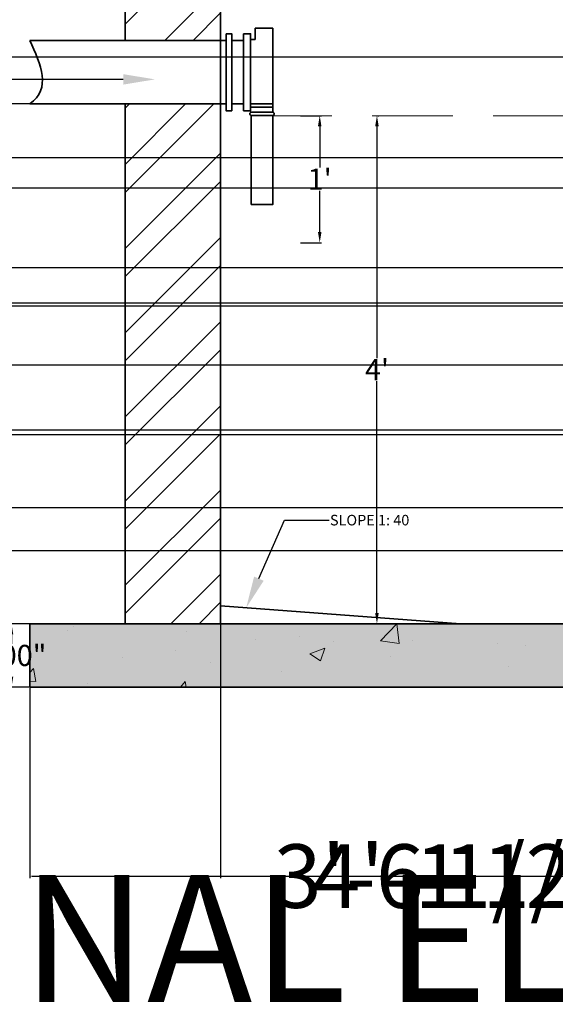
# Model space of a CAD drawing. Units: inches. Extents: x -34 to 285, y -151 to 155.
# Tile 2 of 10: x 22 to 72, y -151 to -58. Entities that reach past the tile are written whole.
import ezdxf
from ezdxf import colors
from ezdxf.entities.mleader import LeaderData, LeaderLine
from ezdxf.math import Vec2, Vec3

# ---------------------------------------------------------------- set-up
doc = ezdxf.new("R2010")
doc.units = ezdxf.units.IN
doc.header["$MEASUREMENT"] = 0
doc.linetypes.add('DASHED', pattern=[19.05, 12.7, -6.35])
for name, color, linetype, lineweight in [('A-ANNO-DIMS', 2, 'Continuous', 18), ('A-ANNO-TEXT', 7, 'Continuous', 25), ('A-DETL', 7, 'Continuous', 35), ('A-DETL-HIDN', 8, 'DASHED', 18), ('A-DETL-PATT', 8, 'Continuous', 18), ('P-SANR-PATT', 8, 'Continuous', 13), ('P-SANR-PIPE', 4, 'Continuous', 35)]:
    doc.layers.add(name, color=color, linetype=linetype, lineweight=lineweight)
doc.styles.get("Standard").update_dxf_attribs({"font": 'arial.ttf'})
doc.dimstyles.get("Standard").update_dxf_attribs({"dimtxt": 6, "dimasz": 0.18, "dimexe": 0.18, "dimexo": 0.0625, "dimgap": 0.09, "dimtad": 0, "dimtih": 1, "dimtoh": 1, "dimzin": 0, "dimdsep": 46, "dimlunit": 3, "dimtxsty": 'Standard', "dimcen": 0.09, "dimadec": 0, "dimazin": 0, "dimtfac": 1, "dimtofl": 0, "dimtmove": 0, "dimatfit": 3, "dimfxl": 1, "dimtolj": 1, "dimtzin": 0, "dimarcsym": 0})
pattern_1 = [(50, (9.538, 3.616), (14.3452, -1.255), [1.5, -16.5]), (355, (9.538, 3.616), (-2.775, 15.0438), [1.2, -13.2]), (100.451, (10.733, 3.511), (11.5702, 13.7888), [1.2748, -14.0228]), (46.184, (9.538, 7.616), (21.345, -3.3104), [2.25, -24.75]), (96.636, (11.317, 7.34), (18.693, 19.4824), [1.912, -21.0343]), (351.184, (9.538, 7.616), (18.693, 19.4824), [1.8, -19.8]), (21, (11.538, 6.616), (11.9381, -8.0524), [1.5, -16.5]), (326, (11.538, 6.616), (4.8663, 14.503), [1.2, -13.2]), (71.451, (12.533, 5.945), (16.8044, 6.4506), [1.2748, -14.0228]), (37.5, (9.538, 3.616), (0.2432, 6.65788), [0, -13.04, 0, -13.4, 0, -13.25]), (7.5, (9.538, 3.616), (5.2614, 7.88823), [0, -7.64, 0, -12.74, 0, -5.05]), (327.5, (5.078, 3.616), (10.67645, -0.4511), [0, -5, 0, -15.6, 0, -20.7]), (317.5, (3.078, 3.616), (11.6637, 2.0021), [0, -6.5, 0, -10.36, 0, -14.7])]

# ---------------------------------------------------------------- blocks, each defined once
blk = doc.blocks.new('*D26')
at = {"layer": 'A-ANNO-DIMS', "color": 0, "lineweight": -2, "transparency": 16777216}
for p, q in [((48.419, -66.969), (50.405, -66.969)), ((50.225, -67.969), (50.225, -71.875)), ((50.225, -77.969), (50.225, -74.063)), ((48.419, -78.969), (50.405, -78.969))]:
    blk.add_line(p, q, dxfattribs=at)
at = {"layer": 'A-ANNO-DIMS', "color": 0, "transparency": 16777216}
for points in [[(50.058, -67.969), (50.391, -67.969), (50.225, -66.969)], [(50.058, -77.969), (50.391, -77.969), (50.225, -78.969)]]:
    blk.add_solid(points, dxfattribs=at)
at = {"layer": 'Defpoints', "color": 0, "transparency": 16777216}
for p in [(48.356, -66.969), (48.356, -78.969), (50.225, -78.969)]:
    blk.add_point(p, dxfattribs=at)
at = {"layer": 'A-ANNO-DIMS', "color": 0, "transparency": 16777216, "insert": (50.225, -72.969), "char_height": 2, "attachment_point": 5}
blk.add_mtext("\\A1;1'", dxfattribs=at)
blk = doc.blocks.new('*D27')
at = {"layer": 'A-ANNO-DIMS', "color": 0, "lineweight": -2, "transparency": 16777216}
for p, q in [((55.697, -66.969), (55.814, -66.969)), ((55.634, -67.969), (55.634, -89.879)), ((55.634, -113.969), (55.634, -92.059)), ((55.697, -114.969), (55.814, -114.969))]:
    blk.add_line(p, q, dxfattribs=at)
at = {"layer": 'A-ANNO-DIMS', "color": 0, "transparency": 16777216}
for points in [[(55.468, -67.969), (55.801, -67.969), (55.634, -66.969)], [(55.468, -113.969), (55.801, -113.969), (55.634, -114.969)]]:
    blk.add_solid(points, dxfattribs=at)
at = {"layer": 'Defpoints', "color": 0, "transparency": 16777216}
for p in [(55.634, -66.969), (55.634, -114.969), (55.634, -114.969)]:
    blk.add_point(p, dxfattribs=at)
at = {"layer": 'A-ANNO-DIMS', "color": 0, "transparency": 16777216, "insert": (55.634, -90.969), "char_height": 2, "attachment_point": 5}
blk.add_mtext("\\A1;4'", dxfattribs=at)
blk = doc.blocks.new('*D35')
at = {"layer": 'A-ANNO-DIMS', "color": 0, "lineweight": -2, "transparency": 16777216}
for p, q in [((21.5, -42.969), (13.144, -42.969)), ((13.324, -43.969), (13.324, -80.858)), ((13.324, -119.969), (13.324, -83.08)), ((22.783, -120.969), (13.144, -120.969))]:
    blk.add_line(p, q, dxfattribs=at)
at = {"layer": 'A-ANNO-DIMS', "color": 0, "transparency": 16777216}
for points in [[(13.157, -43.969), (13.491, -43.969), (13.324, -42.969)], [(13.157, -119.969), (13.491, -119.969), (13.324, -120.969)]]:
    blk.add_solid(points, dxfattribs=at)
at = {"layer": 'Defpoints', "color": 0, "transparency": 16777216}
for p in [(13.324, -42.969), (21.563, -42.969), (22.846, -120.969)]:
    blk.add_point(p, dxfattribs=at)
at = {"layer": 'A-ANNO-DIMS', "color": 0, "transparency": 16777216, "insert": (13.324, -81.969), "char_height": 2, "attachment_point": 5}
blk.add_mtext('\\A1;6\'-6.00"', dxfattribs=at)
blk = doc.blocks.new('*D37')
at = {"layer": 'A-ANNO-DIMS', "color": 0, "lineweight": -2, "transparency": 16777216}
for p, q in [((22.783, -114.969), (20.931, -114.969)), ((21.111, -115.969), (21.111, -116.858)), ((21.111, -119.969), (21.111, -119.08)), ((22.783, -120.969), (20.931, -120.969))]:
    blk.add_line(p, q, dxfattribs=at)
at = {"layer": 'A-ANNO-DIMS', "color": 0, "transparency": 16777216}
for points in [[(20.944, -115.969), (21.278, -115.969), (21.111, -114.969)], [(20.944, -119.969), (21.278, -119.969), (21.111, -120.969)]]:
    blk.add_solid(points, dxfattribs=at)
at = {"layer": 'Defpoints', "color": 0, "transparency": 16777216}
for p in [(22.846, -114.969), (21.111, -120.969), (22.846, -120.969)]:
    blk.add_point(p, dxfattribs=at)
at = {"layer": 'A-ANNO-DIMS', "color": 0, "transparency": 16777216, "insert": (21.111, -117.969), "char_height": 2, "attachment_point": 5}
blk.add_mtext('\\A1;6.00"', dxfattribs=at)
blk = doc.blocks.new('PIPE-SOCKET')
for p, q in [((1.802, 8.25), (0.129, 8.25)), ((1.802, 7.168), (1.802, 8.25)), ((2.233, 7.168), (1.802, 7.168)), ((2.233, 7.168), (2.233, 7.168))]:
    blk.add_line(p, q)
for points in [[(0.129, 0.312), (0.129, 8.25), (1.802, 8.25)], [(0.129, 0.312), (2.172, 0.312)]]:
    blk.add_lwpolyline(points)
for centre, start, end in [((0.157, 0.157), 100.54101, 280.54101), ((2.144, 0.157), 259.45899, 79.45899)]:
    blk.add_arc(centre, 0.157, start, end)
blk = doc.blocks.new('*D48')
at = {"layer": 'A-ANNO-DIMS', "color": 0, "lineweight": -2, "transparency": 16777216}
for p, q in [((22.846, -121.031), (22.846, -138.999)), ((214.846, -121.031), (214.846, -138.999)), ((23.026, -138.819), (108.733, -138.819)), ((214.666, -138.819), (128.959, -138.819))]:
    blk.add_line(p, q, dxfattribs=at)
at = {"layer": 'A-ANNO-DIMS', "color": 0, "transparency": 16777216}
for points in [[(23.026, -138.789), (23.026, -138.849), (22.846, -138.819)], [(214.666, -138.789), (214.666, -138.849), (214.846, -138.819)]]:
    blk.add_solid(points, dxfattribs=at)
at = {"layer": 'Defpoints', "color": 0, "transparency": 16777216}
for p in [(22.846, -120.969), (214.846, -120.969), (214.846, -138.819)]:
    blk.add_point(p, dxfattribs=at)
at = {"layer": 'A-ANNO-DIMS', "color": 0, "transparency": 16777216, "insert": (118.846, -138.819), "char_height": 6, "attachment_point": 5}
blk.add_mtext('\\A1;16\'-0"', dxfattribs=at)
blk = doc.blocks.new('*D57')
at = {"layer": 'A-ANNO-DIMS', "color": 0, "lineweight": -2, "transparency": 16777216}
for p, q in [((41.321, -65.853), (0.722, -65.853)), ((0.902, -66.033), (0.902, -87.309)), ((0.902, -114.789), (0.902, -93.513)), ((40.783, -114.969), (0.722, -114.969))]:
    blk.add_line(p, q, dxfattribs=at)
at = {"layer": 'A-ANNO-DIMS', "color": 0, "transparency": 16777216}
for points in [[(0.872, -66.033), (0.932, -66.033), (0.902, -65.853)], [(0.872, -114.789), (0.932, -114.789), (0.902, -114.969)]]:
    blk.add_solid(points, dxfattribs=at)
at = {"layer": 'Defpoints', "color": 0, "transparency": 16777216}
for p in [(41.384, -65.853), (0.902, -114.969), (40.846, -114.969)]:
    blk.add_point(p, dxfattribs=at)
at = {"layer": 'A-ANNO-DIMS', "color": 0, "transparency": 16777216, "insert": (0.902, -90.411), "char_height": 6, "attachment_point": 5}
blk.add_mtext('\\A1;4\'-1"', dxfattribs=at)
blk = doc.blocks.new('*D58')
at = {"layer": 'A-ANNO-DIMS', "color": 0, "lineweight": -2, "transparency": 16777216}
for p, q in [((83.099, -61.477), (83.099, -138.999)), ((40.846, -115.031), (40.846, -138.999)), ((41.026, -138.819), (46.919, -138.819)), ((82.919, -138.819), (77.026, -138.819))]:
    blk.add_line(p, q, dxfattribs=at)
at = {"layer": 'A-ANNO-DIMS', "color": 0, "transparency": 16777216}
for points in [[(41.026, -138.789), (41.026, -138.849), (40.846, -138.819)], [(82.919, -138.789), (82.919, -138.849), (83.099, -138.819)]]:
    blk.add_solid(points, dxfattribs=at)
at = {"layer": 'Defpoints', "color": 0, "transparency": 16777216}
for p in [(83.099, -61.415), (40.846, -114.969), (83.099, -138.819)]:
    blk.add_point(p, dxfattribs=at)
at = {"layer": 'A-ANNO-DIMS', "color": 0, "transparency": 16777216, "insert": (61.973, -138.819), "char_height": 6, "attachment_point": 5}
blk.add_mtext('\\A1;3\'-6 1/2"', dxfattribs=at)
blk = doc.blocks.new('*D60')
at = {"layer": 'A-ANNO-DIMS', "color": 0, "lineweight": -2, "transparency": 16777216}
for p, q in [((90.383, -71.009), (90.383, -138.999)), ((40.846, -115.031), (40.846, -138.999)), ((41.026, -138.819), (50.439, -138.819)), ((90.203, -138.819), (80.791, -138.819))]:
    blk.add_line(p, q, dxfattribs=at)
at = {"layer": 'A-ANNO-DIMS', "color": 0, "transparency": 16777216}
for points in [[(41.026, -138.789), (41.026, -138.849), (40.846, -138.819)], [(90.203, -138.789), (90.203, -138.849), (90.383, -138.819)]]:
    blk.add_solid(points, dxfattribs=at)
at = {"layer": 'Defpoints', "color": 0, "transparency": 16777216}
for p in [(90.383, -70.947), (40.846, -114.969), (90.383, -138.819)]:
    blk.add_point(p, dxfattribs=at)
at = {"layer": 'A-ANNO-DIMS', "color": 0, "transparency": 16777216, "insert": (65.615, -138.819), "char_height": 6, "attachment_point": 5}
blk.add_mtext('\\A1;4\'-1 1/2"', dxfattribs=at)
blk = doc.blocks.new('*D64')
at = {"layer": 'A-ANNO-DIMS', "color": 0, "lineweight": -2, "transparency": 16777216}
for p, q in [((157.783, -84.969), (0.722, -84.969)), ((0.902, -85.149), (0.902, -96.816)), ((0.902, -114.789), (0.902, -103.122)), ((148.783, -114.969), (0.722, -114.969))]:
    blk.add_line(p, q, dxfattribs=at)
at = {"layer": 'A-ANNO-DIMS', "color": 0, "transparency": 16777216}
for points in [[(0.872, -85.149), (0.932, -85.149), (0.902, -84.969)], [(0.872, -114.789), (0.932, -114.789), (0.902, -114.969)]]:
    blk.add_solid(points, dxfattribs=at)
at = {"layer": 'Defpoints', "color": 0, "transparency": 16777216}
for p in [(157.846, -84.969), (0.902, -114.969), (148.846, -114.969)]:
    blk.add_point(p, dxfattribs=at)
at = {"layer": 'A-ANNO-DIMS', "color": 0, "transparency": 16777216, "insert": (0.902, -99.969), "char_height": 6, "attachment_point": 5}
blk.add_mtext('\\A1;2\'-6"', dxfattribs=at)
blk = doc.blocks.new('*D67')
at = {"layer": 'A-ANNO-DIMS', "color": 0, "lineweight": -2, "transparency": 16777216}
for p, q in [((90.321, -70.947), (0.722, -70.947)), ((0.902, -71.127), (0.902, -89.802)), ((0.902, -114.789), (0.902, -96.113)), ((118.783, -114.969), (0.722, -114.969))]:
    blk.add_line(p, q, dxfattribs=at)
at = {"layer": 'A-ANNO-DIMS', "color": 0, "transparency": 16777216}
for points in [[(0.872, -71.127), (0.932, -71.127), (0.902, -70.947)], [(0.872, -114.789), (0.932, -114.789), (0.902, -114.969)]]:
    blk.add_solid(points, dxfattribs=at)
at = {"layer": 'Defpoints', "color": 0, "transparency": 16777216}
for p in [(90.383, -70.947), (0.902, -114.969), (118.846, -114.969)]:
    blk.add_point(p, dxfattribs=at)
at = {"layer": 'A-ANNO-DIMS', "color": 0, "transparency": 16777216, "insert": (0.902, -92.958), "char_height": 6, "attachment_point": 5}
blk.add_mtext('\\A1;3\'-8"', dxfattribs=at)
blk = doc.blocks.new('*D72')
at = {"layer": 'A-ANNO-DIMS', "color": 0, "lineweight": -2, "transparency": 16777216}
for p, q in [((90.321, -70.947), (0.722, -70.947)), ((0.902, -71.127), (0.902, -72.953)), ((0.902, -81.165), (0.902, -79.338)), ((97.605, -81.345), (0.722, -81.345))]:
    blk.add_line(p, q, dxfattribs=at)
at = {"layer": 'A-ANNO-DIMS', "color": 0, "transparency": 16777216}
for points in [[(0.872, -71.127), (0.932, -71.127), (0.902, -70.947)], [(0.872, -81.165), (0.932, -81.165), (0.902, -81.345)]]:
    blk.add_solid(points, dxfattribs=at)
at = {"layer": 'Defpoints', "color": 0, "transparency": 16777216}
for p in [(90.383, -70.947), (0.902, -81.345), (97.668, -81.345)]:
    blk.add_point(p, dxfattribs=at)
at = {"layer": 'A-ANNO-DIMS', "color": 0, "transparency": 16777216, "insert": (0.902, -76.146), "char_height": 6, "attachment_point": 5}
blk.add_mtext('\\A1;0\'-10 1/2"', dxfattribs=at)
blk = doc.blocks.new('*D73')
at = {"layer": 'A-ANNO-DIMS', "color": 0, "lineweight": -2, "transparency": 16777216}
for p, q in [((97.605, -81.345), (0.722, -81.345)), ((0.902, -81.525), (0.902, -82.784)), ((0.902, -90.35), (0.902, -89.091)), ((105.236, -90.53), (0.722, -90.53))]:
    blk.add_line(p, q, dxfattribs=at)
at = {"layer": 'A-ANNO-DIMS', "color": 0, "transparency": 16777216}
for points in [[(0.872, -81.525), (0.932, -81.525), (0.902, -81.345)], [(0.872, -90.35), (0.932, -90.35), (0.902, -90.53)]]:
    blk.add_solid(points, dxfattribs=at)
at = {"layer": 'Defpoints', "color": 0, "transparency": 16777216}
for p in [(97.668, -81.345), (0.902, -90.53), (105.299, -90.53)]:
    blk.add_point(p, dxfattribs=at)
at = {"layer": 'A-ANNO-DIMS', "color": 0, "transparency": 16777216, "insert": (0.902, -85.937), "char_height": 6, "attachment_point": 5}
blk.add_mtext('\\A1;0\'-9"', dxfattribs=at)
blk = doc.blocks.new('*D74')
at = {"layer": 'A-ANNO-DIMS', "color": 0, "lineweight": -2, "transparency": 16777216}
for p, q in [((0.902, -90.35), (0.902, -90.17)), ((105.236, -90.53), (0.722, -90.53)), ((115.989, -97.116), (0.722, -97.116)), ((0.902, -97.296), (0.902, -97.476))]:
    blk.add_line(p, q, dxfattribs=at)
at = {"layer": 'A-ANNO-DIMS', "color": 0, "transparency": 16777216}
for points in [[(0.872, -90.35), (0.932, -90.35), (0.902, -90.53)], [(0.872, -97.296), (0.932, -97.296), (0.902, -97.116)]]:
    blk.add_solid(points, dxfattribs=at)
at = {"layer": 'Defpoints', "color": 0, "transparency": 16777216}
for p in [(105.299, -90.53), (0.902, -97.116), (116.051, -97.116)]:
    blk.add_point(p, dxfattribs=at)
at = {"layer": 'A-ANNO-DIMS', "color": 0, "transparency": 16777216, "insert": (0.902, -93.823), "char_height": 6, "attachment_point": 5}
blk.add_mtext('\\A1;0\'-6 1/2"', dxfattribs=at)
blk = doc.blocks.new('*D75')
at = {"layer": 'A-ANNO-DIMS', "color": 0, "lineweight": -2, "transparency": 16777216}
for p, q in [((115.989, -97.116), (0.722, -97.116)), ((0.902, -97.296), (0.902, -97.419)), ((121.836, -104.028), (0.722, -104.028)), ((0.902, -103.848), (0.902, -103.725))]:
    blk.add_line(p, q, dxfattribs=at)
at = {"layer": 'A-ANNO-DIMS', "color": 0, "transparency": 16777216}
for points in [[(0.872, -97.296), (0.932, -97.296), (0.902, -97.116)], [(0.872, -103.848), (0.932, -103.848), (0.902, -104.028)]]:
    blk.add_solid(points, dxfattribs=at)
at = {"layer": 'Defpoints', "color": 0, "transparency": 16777216}
for p in [(116.051, -97.116), (0.902, -104.028), (121.899, -104.028)]:
    blk.add_point(p, dxfattribs=at)
at = {"layer": 'A-ANNO-DIMS', "color": 0, "transparency": 16777216, "insert": (0.902, -100.572), "char_height": 6, "attachment_point": 5}
blk.add_mtext('\\A1;0\'-7"', dxfattribs=at)
blk = doc.blocks.new('*D76')
at = {"layer": 'A-ANNO-DIMS', "color": 0, "lineweight": -2, "transparency": 16777216}
for p, q in [((121.836, -104.028), (0.722, -104.028)), ((0.902, -104.208), (0.902, -106.345)), ((0.902, -114.789), (0.902, -112.652)), ((118.783, -114.969), (0.722, -114.969))]:
    blk.add_line(p, q, dxfattribs=at)
at = {"layer": 'A-ANNO-DIMS', "color": 0, "transparency": 16777216}
for points in [[(0.872, -104.208), (0.932, -104.208), (0.902, -104.028)], [(0.872, -114.789), (0.932, -114.789), (0.902, -114.969)]]:
    blk.add_solid(points, dxfattribs=at)
at = {"layer": 'Defpoints', "color": 0, "transparency": 16777216}
for p in [(121.899, -104.028), (0.902, -114.969), (118.846, -114.969)]:
    blk.add_point(p, dxfattribs=at)
at = {"layer": 'A-ANNO-DIMS', "color": 0, "transparency": 16777216, "insert": (0.902, -109.499), "char_height": 6, "attachment_point": 5}
blk.add_mtext('\\A1;0\'-11"', dxfattribs=at)
blk = doc.blocks.new('*D83')
at = {"layer": 'A-ANNO-DIMS', "color": 0, "lineweight": -2, "transparency": 16777216}
for p, q in [((153.652, -61.451), (0.722, -61.451)), ((0.902, -61.631), (0.902, -64.435)), ((0.902, -73.623), (0.902, -70.819)), ((162.652, -73.803), (0.722, -73.803))]:
    blk.add_line(p, q, dxfattribs=at)
at = {"layer": 'A-ANNO-DIMS', "color": 0, "transparency": 16777216}
for points in [[(0.872, -61.631), (0.932, -61.631), (0.902, -61.451)], [(0.872, -73.623), (0.932, -73.623), (0.902, -73.803)]]:
    blk.add_solid(points, dxfattribs=at)
at = {"layer": 'Defpoints', "color": 0, "transparency": 16777216}
for p in [(153.715, -61.451), (0.902, -73.803), (162.715, -73.803)]:
    blk.add_point(p, dxfattribs=at)
at = {"layer": 'A-ANNO-DIMS', "color": 0, "transparency": 16777216, "insert": (0.902, -67.627), "char_height": 6, "attachment_point": 5}
blk.add_mtext('\\A1;1\'-0 1/2"', dxfattribs=at)
blk = doc.blocks.new('*D84')
at = {"layer": 'A-ANNO-DIMS', "color": 0, "lineweight": -2, "transparency": 16777216}
for p, q in [((162.652, -73.803), (0.722, -73.803)), ((0.902, -73.983), (0.902, -76.094)), ((0.902, -84.513), (0.902, -82.401)), ((169.24, -84.693), (0.722, -84.693))]:
    blk.add_line(p, q, dxfattribs=at)
at = {"layer": 'A-ANNO-DIMS', "color": 0, "transparency": 16777216}
for points in [[(0.872, -73.983), (0.932, -73.983), (0.902, -73.803)], [(0.872, -84.513), (0.932, -84.513), (0.902, -84.693)]]:
    blk.add_solid(points, dxfattribs=at)
at = {"layer": 'Defpoints', "color": 0, "transparency": 16777216}
for p in [(162.715, -73.803), (0.902, -84.693), (169.303, -84.693)]:
    blk.add_point(p, dxfattribs=at)
at = {"layer": 'A-ANNO-DIMS', "color": 0, "transparency": 16777216, "insert": (0.902, -79.248), "char_height": 6, "attachment_point": 5}
blk.add_mtext('\\A1;0\'-11"', dxfattribs=at)
blk = doc.blocks.new('*D85')
at = {"layer": 'A-ANNO-DIMS', "color": 0, "lineweight": -2, "transparency": 16777216}
for p, q in [((169.24, -84.693), (0.722, -84.693)), ((0.902, -84.873), (0.902, -87.539)), ((0.902, -96.513), (0.902, -93.846)), ((179.419, -96.693), (0.722, -96.693))]:
    blk.add_line(p, q, dxfattribs=at)
at = {"layer": 'A-ANNO-DIMS', "color": 0, "transparency": 16777216}
for points in [[(0.872, -84.873), (0.932, -84.873), (0.902, -84.693)], [(0.872, -96.513), (0.932, -96.513), (0.902, -96.693)]]:
    blk.add_solid(points, dxfattribs=at)
at = {"layer": 'Defpoints', "color": 0, "transparency": 16777216}
for p in [(169.303, -84.693), (0.902, -96.693), (179.482, -96.693)]:
    blk.add_point(p, dxfattribs=at)
at = {"layer": 'A-ANNO-DIMS', "color": 0, "transparency": 16777216, "insert": (0.902, -90.693), "char_height": 6, "attachment_point": 5}
blk.add_mtext('\\A1;1\'-0"', dxfattribs=at)
blk = doc.blocks.new('*D86')
at = {"layer": 'A-ANNO-DIMS', "color": 0, "lineweight": -2, "transparency": 16777216}
for p, q in [((179.419, -96.693), (0.722, -96.693)), ((0.902, -96.873), (0.902, -99.189)), ((0.902, -107.89), (0.902, -105.574)), ((187.783, -108.07), (0.722, -108.07))]:
    blk.add_line(p, q, dxfattribs=at)
at = {"layer": 'A-ANNO-DIMS', "color": 0, "transparency": 16777216}
for points in [[(0.872, -96.873), (0.932, -96.873), (0.902, -96.693)], [(0.872, -107.89), (0.932, -107.89), (0.902, -108.07)]]:
    blk.add_solid(points, dxfattribs=at)
at = {"layer": 'Defpoints', "color": 0, "transparency": 16777216}
for p in [(179.482, -96.693), (0.902, -108.07), (187.846, -108.07)]:
    blk.add_point(p, dxfattribs=at)
at = {"layer": 'A-ANNO-DIMS', "color": 0, "transparency": 16777216, "insert": (0.902, -102.381), "char_height": 6, "attachment_point": 5}
blk.add_mtext('\\A1;0\'-11 1/2"', dxfattribs=at)
blk = doc.blocks.new('*D87')
at = {"layer": 'A-ANNO-DIMS', "color": 0, "lineweight": -2, "transparency": 16777216}
for p, q in [((187.783, -108.07), (0.722, -108.07)), ((0.902, -108.25), (0.902, -108.366)), ((196.783, -114.969), (0.722, -114.969)), ((0.902, -114.789), (0.902, -114.673))]:
    blk.add_line(p, q, dxfattribs=at)
at = {"layer": 'A-ANNO-DIMS', "color": 0, "transparency": 16777216}
for points in [[(0.872, -108.25), (0.932, -108.25), (0.902, -108.07)], [(0.872, -114.789), (0.932, -114.789), (0.902, -114.969)]]:
    blk.add_solid(points, dxfattribs=at)
at = {"layer": 'Defpoints', "color": 0, "transparency": 16777216}
for p in [(187.846, -108.07), (0.902, -114.969), (196.846, -114.969)]:
    blk.add_point(p, dxfattribs=at)
at = {"layer": 'A-ANNO-DIMS', "color": 0, "transparency": 16777216, "insert": (0.902, -111.519), "char_height": 6, "attachment_point": 5}
blk.add_mtext('\\A1;0\'-7"', dxfattribs=at)

msp = doc.modelspace()

# ---------------------------------------------------------------- hatches: boundary and pattern name
at = {"layer": 'A-DETL-PATT'}
h = msp.add_hatch(dxfattribs=at)
h.set_pattern_fill('AR-CONC', color=256, scale=0.4)
h.set_pattern_definition([(50, (0, 0), (2.86904, -0.251009), [0.3, -3.3]), (355, (0, 0), (-0.555005, 3.00877), [0.24, -2.64]), (100.4514, (0.239, -0.021), (2.314035, 2.75776), [0.25496, -2.80457]), (46.1842, (0, 0.8), (4.268965, -0.662077), [0.45, -4.95]), (96.6356, (0.3557, 0.745), (3.73865, 3.896474), [0.38244, -4.206855]), (351.1842, (0, 0.8), (3.73865, 3.896474), [0.36, -3.96]), (21, (0.4, 0.6), (2.387628, -1.610476), [0.3, -3.3]), (326, (0.4, 0.6), (0.97326, 2.9006), [0.24, -2.64]), (71.4514, (0.599, 0.4658), (3.36089, 1.290125), [0.25496, -2.80457]), (37.5, (0, 0), (0.0486394, 1.3315754), [0, -2.608, 0, -2.68, 0, -2.65]), (7.5, (0, 0), (1.052278, 1.577647), [0, -1.528, 0, -2.548, 0, -1.01]), (327.5, (-0.892, 0), (2.1352897, -0.0902195), [0, -1, 0, -3.12, 0, -4.14]), (317.5, (-1.292, 0), (2.332745, 0.40042), [0, -1.3, 0, -2.072, 0, -2.94])])
h.paths.add_polyline_path([(214.846, -48.969), (214.846, -42.969), (184.518, -42.969), (184.518, -48.969)])
h.paths.add_polyline_path([(122.241, -42.969), (122.241, -48.969), (155.156, -48.969), (155.156, -42.969)])
h.paths.add_polyline_path([(214.846, -114.969), (22.846, -114.969), (22.846, -120.969), (214.846, -120.969)])
h = msp.add_hatch(dxfattribs=at)
h.set_pattern_fill('ANSI32', color=256, scale=15)
h.paths.add_polyline_path([(148.846, -59.969), (139.846, -59.969), (139.846, -66.969), (148.846, -66.969)])
h.paths.add_polyline_path([(148.846, -66.969), (139.846, -66.969), (139.846, -78.969), (148.846, -78.969)])
h.paths.add_polyline_path([(148.846, -84.969), (139.846, -84.969), (139.846, -85.88), (139.846, -114.969), (148.846, -114.969)])
h.paths.add_polyline_path([(40.846, -65.853), (32.384, -65.853), (31.846, -65.853), (31.846, -114.969), (40.846, -114.969)])
h.paths.add_polyline_path([(40.846, -48.969), (31.846, -48.969), (31.846, -59.853), (40.846, -59.853)])
h = msp.add_hatch(dxfattribs=at)
h.set_pattern_fill('AR-CONC', color=256, scale=2)
h.paths.add_polyline_path([(22.846, -114.969), (22.846, -120.969), (214.846, -120.969), (214.846, -114.969)])
at = {"layer": 'P-SANR-PATT'}
h = msp.add_hatch(dxfattribs=at)
h.set_pattern_fill('AR-CONC', color=256, scale=2)
h.set_pattern_definition(pattern_1)
h.paths.add_polyline_path([(41.921, -59.235), (41.384, -59.235), (41.384, -66.504), (41.921, -66.504)])
h.paths.add_polyline_path([(43.693, -59.235), (43.04, -59.235), (43.04, -66.504), (43.693, -66.504)])
h = msp.add_hatch(dxfattribs=at)
h.set_pattern_fill('AR-CONC', color=256, scale=2)
h.set_pattern_definition(pattern_1)
h.paths.add_polyline_path([(45.798, -66.948, 0.831086), (45.798, -66.639), (43.754, -66.639, 0.831086), (43.754, -66.948)])
h = msp.add_hatch(dxfattribs=at)
h.set_pattern_fill('AR-CONC', color=256, scale=2)
h.paths.add_polyline_path([(34.155, -69.469), (36.26, -69.469), (36.26, -69.778), (34.155, -69.778)])

# ---------------------------------------------------------------- linework, layer by layer
at = {"layer": 'A-DETL'}
for p, q in [((31.846, -48.969), (31.846, -59.853)), ((40.846, -48.969), (40.846, -114.969)), ((31.846, -65.853), (31.846, -114.969)), ((40.846, -113.284), (63.519, -114.969)), ((22.846, -114.969), (22.846, -120.969)), ((22.846, -114.969), (214.846, -114.969)), ((22.846, -120.969), (214.846, -120.969))]:
    msp.add_line(p, q, dxfattribs=at)
at = {"layer": 'A-DETL-HIDN', "ltscale": 0.6}
msp.add_line((43.754, -66.969), (73.547, -66.969), dxfattribs=at)
at = {"layer": 'P-SANR-PIPE'}
for p, q in [((41.384, -59.853), (22.832, -59.853)), ((41.384, -59.853), (32.384, -59.853)), ((41.384, -65.853), (22.832, -65.853)), ((41.384, -65.853), (23.384, -65.853)), ((41.384, -65.853), (32.384, -65.853)), ((43.04, -65.853), (41.921, -65.853)), ((45.798, -75.353), (43.754, -75.353))]:
    msp.add_line(p, q, dxfattribs=at)
for points in [[(41.384, -59.235), (41.921, -59.235), (41.921, -66.504), (41.384, -66.504)], [(43.04, -59.235), (43.693, -59.235), (43.693, -66.504), (43.04, -66.504)], [(41.921, -59.853), (43.04, -59.853), (43.04, -65.853), (41.921, -65.853)]]:
    msp.add_lwpolyline(points, close=True, dxfattribs=at)
for points in [[(32.384, -59.853), (22.832, -59.853)], [(22.832, -65.853), (32.384, -65.853)], [(43.693, -66.162), (45.798, -66.162), (45.798, -65.853), (43.754, -65.853)], [(43.754, -66.948), (43.754, -75.353), (45.798, -75.353), (45.798, -66.948)], [(43.754, -66.948), (45.798, -66.948)]]:
    msp.add_lwpolyline(points, dxfattribs=at)
msp.add_open_spline([(22.832, -59.853), (23.874, -62.138), (24.916, -64.424), (22.832, -65.853)], degree=3, dxfattribs=at)

# ---------------------------------------------------------------- block references
at = {"layer": 'P-SANR-PIPE', "extrusion": (0, 0, -1), "zscale": -1}
msp.add_blockref('PIPE-SOCKET', (-45.926, -66.951), dxfattribs=at)

# ---------------------------------------------------------------- texts
at = {"layer": 'A-ANNO-TEXT', "insert": (-34.52, -138.72), "char_height": 12, "attachment_point": 1}
msp.add_mtext_dynamic_manual_height_columns('SECTIONAL ELEVATION OF A SEPTIC TANK ', width=509.35271, gutter_width=1, heights=[0], dxfattribs=at)

# ---------------------------------------------------------------- dimensions: what is measured, and where the dimension line sits
at = {"layer": 'A-ANNO-DIMS'}
for base, p1, p2, override, picture, middle in [((13.324, -42.969), (22.846, -120.969), (21.563, -42.969), {"dimtxt": 2, "dimasz": 1, "dimclrd": 0, "dimclre": 0, "dimclrt": 0}, '*D35', (13.324, -81.969)), ((0.902, -73.803), (153.715, -61.451), (162.715, -73.803), {"dimdec": 1, "dimlfac": 1, "dimrnd": 0, "dimzin": 1, "dimdsep": 46, "dimlunit": 4, "dimfrac": 2}, '*D83', (0.902, -67.627)), ((0.902, -114.969), (41.384, -65.853), (40.846, -114.969), {"dimdec": 1, "dimlfac": 1, "dimrnd": 0, "dimzin": 1, "dimdsep": 46, "dimlunit": 4, "dimfrac": 2}, '*D57', (0.902, -90.411)), ((50.225, -78.969), (48.356, -66.969), (48.356, -78.969), {"dimtxt": 2, "dimasz": 1, "dimclrd": 0, "dimclre": 0, "dimclrt": 0}, '*D26', (50.225, -72.969)), ((55.634, -114.969), (55.634, -66.969), (55.634, -114.969), {"dimtxt": 2, "dimasz": 1, "dimclrd": 0, "dimclre": 0, "dimclrt": 0}, '*D27', (55.634, -90.969)), ((0.902, -81.345), (90.383, -70.947), (97.668, -81.345), {"dimdec": 1, "dimlfac": 1, "dimrnd": 0, "dimzin": 1, "dimdsep": 46, "dimlunit": 4, "dimfrac": 2}, '*D72', (0.902, -76.146)), ((0.902, -114.969), (90.383, -70.947), (118.846, -114.969), {"dimdec": 1, "dimlfac": 1, "dimrnd": 0, "dimzin": 1, "dimdsep": 46, "dimlunit": 4, "dimfrac": 2}, '*D67', (0.902, -92.958)), ((0.902, -84.693), (162.715, -73.803), (169.303, -84.693), {"dimdec": 1, "dimlfac": 1, "dimrnd": 0, "dimzin": 1, "dimdsep": 46, "dimlunit": 4, "dimfrac": 2}, '*D84', (0.902, -79.248)), ((0.902, -90.53), (97.668, -81.345), (105.299, -90.53), {"dimdec": 1, "dimlfac": 1, "dimrnd": 0, "dimzin": 1, "dimdsep": 46, "dimlunit": 4, "dimfrac": 2}, '*D73', (0.902, -85.937)), ((0.902, -97.116), (105.299, -90.53), (116.051, -97.116), {"dimdec": 1, "dimlfac": 1, "dimrnd": 0, "dimzin": 1, "dimdsep": 46, "dimlunit": 4, "dimfrac": 2}, '*D74', (0.902, -93.823)), ((0.902, -96.693), (169.303, -84.693), (179.482, -96.693), {"dimdec": 1, "dimlfac": 1, "dimrnd": 0, "dimzin": 1, "dimdsep": 46, "dimlunit": 4, "dimfrac": 2}, '*D85', (0.902, -90.693)), ((0.902, -114.969), (157.846, -84.969), (148.846, -114.969), {"dimdec": 1, "dimlfac": 1, "dimrnd": 0, "dimzin": 1, "dimdsep": 46, "dimlunit": 4, "dimfrac": 2}, '*D64', (0.902, -99.969)), ((0.902, -108.07), (179.482, -96.693), (187.846, -108.07), {"dimdec": 1, "dimlfac": 1, "dimrnd": 0, "dimzin": 1, "dimdsep": 46, "dimlunit": 4, "dimfrac": 2}, '*D86', (0.902, -102.381)), ((0.902, -104.028), (116.051, -97.116), (121.899, -104.028), {"dimdec": 1, "dimlfac": 1, "dimrnd": 0, "dimzin": 1, "dimdsep": 46, "dimlunit": 4, "dimfrac": 2}, '*D75', (0.902, -100.572)), ((0.902, -114.969), (121.899, -104.028), (118.846, -114.969), {"dimdec": 1, "dimlfac": 1, "dimrnd": 0, "dimzin": 1, "dimdsep": 46, "dimlunit": 4, "dimfrac": 2}, '*D76', (0.902, -109.499)), ((0.902, -114.969), (187.846, -108.07), (196.846, -114.969), {"dimdec": 1, "dimlfac": 1, "dimrnd": 0, "dimzin": 1, "dimdsep": 46, "dimlunit": 4, "dimfrac": 2}, '*D87', (0.902, -111.519)), ((21.111, -120.969), (22.846, -114.969), (22.846, -120.969), {"dimtxt": 2, "dimasz": 1, "dimclrd": 0, "dimclre": 0, "dimclrt": 0}, '*D37', (21.111, -117.969))]:
    dim = msp.add_linear_dim(base=base, p1=p1, p2=p2, angle=90, dimstyle='Standard', override=override, dxfattribs=at)
    dim.commit()
    dim.dimension.update_dxf_attribs({"geometry": picture, "text_midpoint": middle})
for base, p1, p2, picture, middle in [((83.099, -138.819), (40.846, -114.969), (83.099, -61.415), '*D58', (61.973, -138.819)), ((90.383, -138.819), (40.846, -114.969), (90.383, -70.947), '*D60', (65.615, -138.819)), ((214.846, -138.819), (22.846, -120.969), (214.846, -120.969), '*D48', (118.846, -138.819))]:
    dim = msp.add_linear_dim(base=base, p1=p1, p2=p2, dimstyle='Standard', override={"dimdec": 1, "dimlfac": 1, "dimrnd": 0, "dimzin": 1, "dimdsep": 46, "dimlunit": 4, "dimfrac": 2}, dxfattribs=at)
    dim.commit()
    dim.dimension.update_dxf_attribs({"geometry": picture, "text_midpoint": middle})

# ---------------------------------------------------------------- leaders
at = {"layer": 'A-ANNO-TEXT'}
ml = msp.add_multileader_mtext('Standard', dxfattribs=at)
ml.set_content('9" THICK BRICK \\PMASONRY ', color=(248, 215, 49))
ml.set_leader_properties()
ml.build(insert=Vec2(0, 0))
ml.multileader.update_dxf_attribs({"dogleg_length": 4.22, "arrow_head_size": 3})
ctx = ml.context
ctx.base_point, ctx.char_height, ctx.arrow_head_size, ctx.landing_gap_size, ctx.plane_origin = Vec3(2.785, -54.411), 1, 3, 0.09, Vec3(31.846, -54.411)
notes = []
notes.append((ctx, [(0, (1, 1, 0), (17.634, -54.411), (-1, 0), 4.22, [(0, [(31.846, -54.411)], 0, [])])]))
ctx.mtext.insert, ctx.mtext.flow_direction = Vec3(2.875, -53.902), 5
ml = msp.add_multileader_mtext('Standard', dxfattribs=at)
ml.set_content('INLET PIPE\\P4" ', color=(248, 215, 49))
ml.set_leader_properties()
ml.build(insert=Vec2(0, 0))
ml.multileader.update_dxf_attribs({"dogleg_length": 4.22, "arrow_head_size": 3})
ctx = ml.context
ctx.base_point, ctx.char_height, ctx.arrow_head_size, ctx.landing_gap_size, ctx.plane_origin = Vec3(2.763, -63.539), 1, 3, 0.09, Vec3(34.669, -63.539)
notes.append((ctx, [(0, (1, 1, 0), (14.489, -63.539), (-1, 0), 4.22, [(0, [(34.669, -63.539)], 0, [])])]))
ctx.mtext.insert, ctx.mtext.flow_direction = Vec3(2.853, -63.039), 5
ml = msp.add_multileader_mtext('Standard', dxfattribs=at)
ml.set_content('SLOPE 1: 40', color=(248, 215, 49))
ml.set_leader_properties()
ml.build(insert=Vec2(0, 0))
ml.multileader.update_dxf_attribs({"dogleg_length": 4.22, "arrow_head_size": 3})
ctx = ml.context
ctx.base_point, ctx.char_height, ctx.arrow_head_size, ctx.landing_gap_size, ctx.plane_origin = Vec3(51.105, -105.192), 1, 3, 0.09, Vec3(43.283, -113.465)
notes.append((ctx, [(0, (1, 1, 0), (46.885, -105.192), (1, 0), 4.22, [(0, [(43.283, -113.465)], 0, [])])]))
ctx.mtext.insert, ctx.mtext.flow_direction = Vec3(51.195, -104.684), 5
for ctx, leaders in notes:
    for number, flags, end, landing, length, lines in leaders:
        leader = LeaderData()
        leader.index, (leader.has_last_leader_line, leader.has_dogleg_vector, leader.attachment_direction) = number, flags
        leader.last_leader_point, leader.dogleg_vector, leader.dogleg_length = Vec3(end), Vec3(landing), length
        for number, points, colour, breaks in lines:
            line = LeaderLine()
            line.index, line.vertices, line.color, line.breaks = number, Vec3.list(points), colors.encode_raw_color(colour), breaks
            leader.lines.append(line)
        ctx.leaders.append(leader)

doc.saveas('drawing.dxf')
